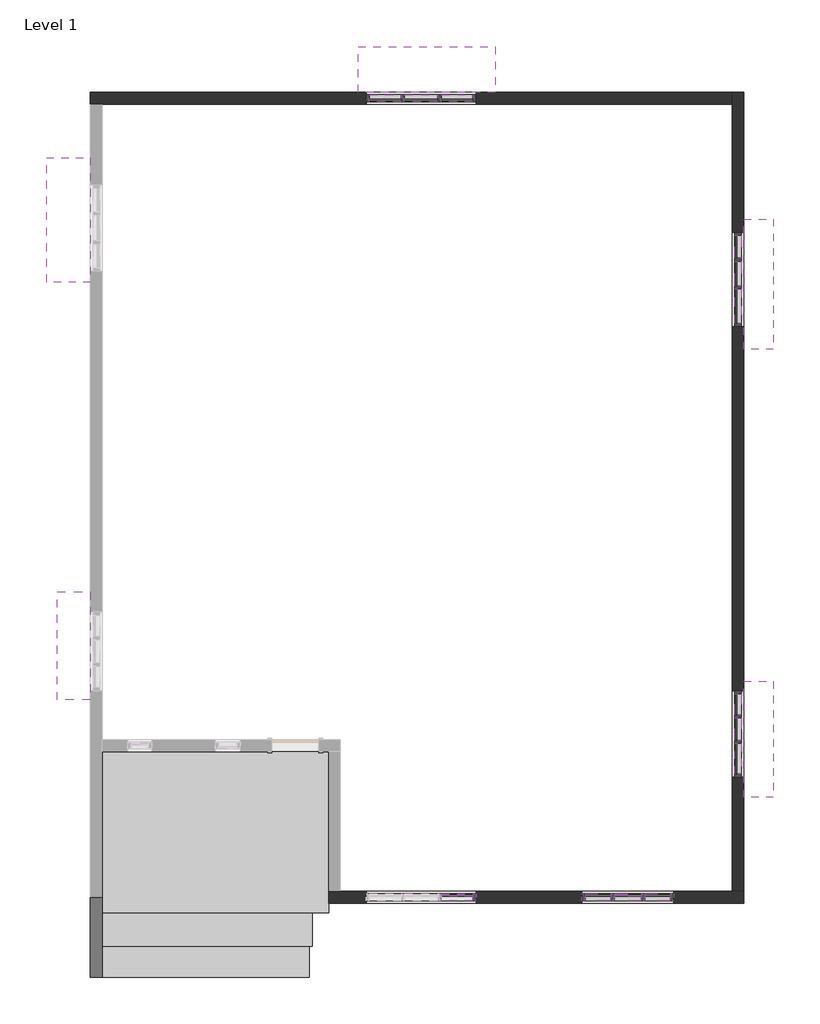
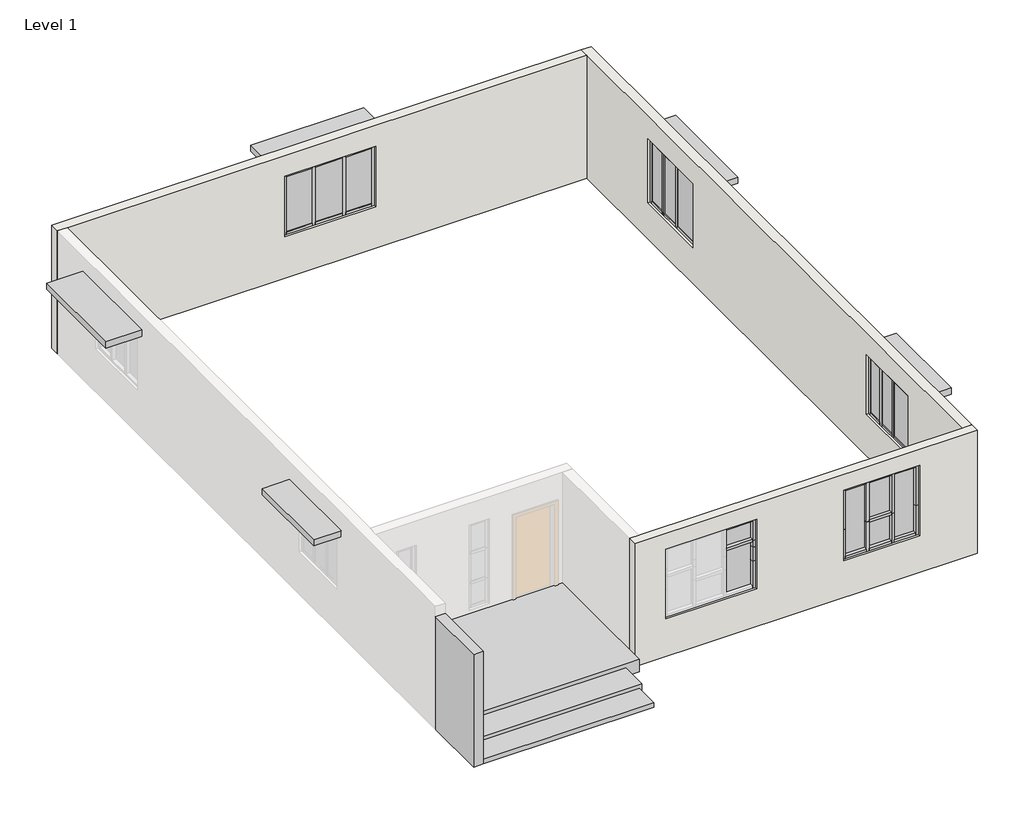
# One storey, part 2 of 2: 51 members, 15 plates, 7 proxies, 3 walls.
"""IFC4 building model written with IfcOpenShell, lengths in millimetres."""

from ifc_helpers import new_model, si_unit, origin, place, context, project, spatial, faceted_brep, transform, mapped, element, save
from components import generic_models_1_generic_models_1_906a804f, generic_models_10_generic_models_10_282af4fe, generic_models_2_generic_models_2_14940448, generic_models_6_generic_models_6_d29c9edd, generic_models_7_generic_models_7_79cca6d0, generic_models_8_generic_models_8_c95dbc8d, generic_models_9_generic_models_9_e403c41d, member_d39130fe, member_be967ef6, member_3f0e0172, member_5215b92c, member_f8dc38bf, member_b3e0441e, member_2caf9219, member_d7af48b5, member_43b2f8c3, member_8ca7f02a, member_b2ed26c7, member_f209f73c, member_fde90c6a, member_7d21ba3d, member_69a911c1, member_1ad5418d, member_e5d39754, member_40abf7f1, member_852981e0, member_2b79973d, member_c33c434a, member_082242e3, member_b4cb8141, member_6fb4a552, member_8bf3bd84, member_143ec642, system_panel_glazed_68735acb, system_panel_glazed_e2a89770, system_panel_glazed_32595814, system_panel_glazed_0cc7d14b, system_panel_glazed_9e372a4a, system_panel_glazed_a8526af5, system_panel_glazed_e1e129e0, system_panel_glazed_32fc5117, system_panel_glazed_c34084c8, system_panel_glazed_d4004c69, system_panel_glazed_e16a1513, system_panel_glazed_7001ef1f, system_panel_glazed_27f6d1d6

model = new_model("IFC4")

# Units and contexts
model_context = context("Model", 3, world=origin())
ifc_project = project(units=[si_unit("LENGTHUNIT", "METRE", prefix="MILLI")], contexts=[model_context])

# Site, building, storey
site = spatial("IfcSite", under=ifc_project)
building = spatial("IfcBuilding", under=site)
storey = spatial("IfcBuildingStorey", under=building, Name="Level 1", Elevation=0.0)

# Proxies
placement = place(None, origin())
generic_models_1_generic_models_1_shape = generic_models_1_generic_models_1_906a804f(model_context)
element("IfcBuildingElementProxy", 1, Name="Generic Models 1 : Generic Models 1", ObjectType="Generic Models 1 : Generic Models 1", at=placement, inside=storey, context=model_context, shape_type="MappedRepresentation", body=[
    mapped(generic_models_1_generic_models_1_shape, transform((0.0, 0.0, 0.0), x_axis=(1.0, 0.0, 0.0), y_axis=(0.0, 1.0, 0.0), z_axis=(0.0, 0.0, 1.0))),
])
generic_models_10_generic_models_10_shape = generic_models_10_generic_models_10_282af4fe(model_context)
element("IfcBuildingElementProxy", 2, Name="Generic Models 10 : Generic Models 10", ObjectType="Generic Models 10 : Generic Models 10", at=placement, inside=storey, context=model_context, shape_type="MappedRepresentation", body=[
    mapped(generic_models_10_generic_models_10_shape, transform((0.0, 0.0, 0.0), x_axis=(1.0, 0.0, 0.0), y_axis=(0.0, 1.0, 0.0), z_axis=(0.0, 0.0, 1.0))),
])
generic_models_2_generic_models_2_shape = generic_models_2_generic_models_2_14940448(model_context)
element("IfcBuildingElementProxy", 3, Name="Generic Models 2 : Generic Models 2", ObjectType="Generic Models 2 : Generic Models 2", at=placement, inside=storey, context=model_context, shape_type="MappedRepresentation", body=[
    mapped(generic_models_2_generic_models_2_shape, transform((0.0, 0.0, 0.0), x_axis=(1.0, 0.0, 0.0), y_axis=(0.0, 1.0, 0.0), z_axis=(0.0, 0.0, 1.0))),
])
generic_models_6_generic_models_6_shape = generic_models_6_generic_models_6_d29c9edd(model_context)
element("IfcBuildingElementProxy", 4, Name="Generic Models 6 : Generic Models 6", ObjectType="Generic Models 6 : Generic Models 6", at=placement, inside=storey, context=model_context, shape_type="MappedRepresentation", body=[
    mapped(generic_models_6_generic_models_6_shape, transform((0.0, 0.0, 0.0), x_axis=(1.0, 0.0, 0.0), y_axis=(0.0, 1.0, 0.0), z_axis=(0.0, 0.0, 1.0))),
])
generic_models_7_generic_models_7_shape = generic_models_7_generic_models_7_79cca6d0(model_context)
element("IfcBuildingElementProxy", 5, Name="Generic Models 7 : Generic Models 7", ObjectType="Generic Models 7 : Generic Models 7", at=placement, inside=storey, context=model_context, shape_type="MappedRepresentation", body=[
    mapped(generic_models_7_generic_models_7_shape, transform((0.0, 0.0, 0.0), x_axis=(1.0, 0.0, 0.0), y_axis=(0.0, 1.0, 0.0), z_axis=(0.0, 0.0, 1.0))),
])
generic_models_8_generic_models_8_shape = generic_models_8_generic_models_8_c95dbc8d(model_context)
element("IfcBuildingElementProxy", 6, Name="Generic Models 8 : Generic Models 8", ObjectType="Generic Models 8 : Generic Models 8", at=placement, inside=storey, context=model_context, shape_type="MappedRepresentation", body=[
    mapped(generic_models_8_generic_models_8_shape, transform((0.0, 0.0, 0.0), x_axis=(1.0, 0.0, 0.0), y_axis=(0.0, 1.0, 0.0), z_axis=(0.0, 0.0, 1.0))),
])
generic_models_9_generic_models_9_shape = generic_models_9_generic_models_9_e403c41d(model_context)
element("IfcBuildingElementProxy", 7, Name="Generic Models 9 : Generic Models 9", ObjectType="Generic Models 9 : Generic Models 9", at=placement, inside=storey, context=model_context, shape_type="MappedRepresentation", body=[
    mapped(generic_models_9_generic_models_9_shape, transform((0.0, 0.0, 0.0), x_axis=(1.0, 0.0, 0.0), y_axis=(0.0, 1.0, 0.0), z_axis=(0.0, 0.0, 1.0))),
])

# Members
member_shape = member_d39130fe(model_context)
element("IfcMember", 8, ObjectType="Rectangular Mullion : 2.5\" x 5\" rectangular", at=placement, inside=storey, context=model_context, shape_type="MappedRepresentation", body=[
    mapped(member_shape, transform((-14378.0161422, -14789.9171312, 1612.541933), x_axis=(1.0, 0.0, 0.0), y_axis=(0.0, -1.0, 0.0), z_axis=(0.0, 0.0, -1.0))),
])
member_2_shape = member_be967ef6(model_context)
element("IfcMember", 9, ObjectType="Rectangular Mullion : 2.5\" x 5\" rectangular", at=placement, inside=storey, context=model_context, shape_type="MappedRepresentation", body=[
    mapped(member_2_shape, transform((-14378.0161422, -14789.9171312, 934.5922675), x_axis=(1.0, 0.0, 0.0), y_axis=(0.0, -1.0, 0.0), z_axis=(0.0, 0.0, -1.0))),
])
member_3_shape = member_3f0e0172(model_context)
element("IfcMember", 10, ObjectType="Rectangular Mullion : 2.5\" x 5\" rectangular", at=placement, inside=storey, context=model_context, shape_type="MappedRepresentation", body=[
    mapped(member_3_shape, transform((-15832.1661422, 678.6828688, 1031.9141224), x_axis=(0.0, 0.0, -1.0), y_axis=(0.0, 1.0, 0.0), z_axis=(1.0, 0.0, 0.0))),
])
element("IfcMember", 11, ObjectType="Rectangular Mullion : 2.5\" x 5\" rectangular", at=placement, inside=storey, context=model_context, shape_type="MappedRepresentation", body=[
    mapped(member_3_shape, transform((-14441.5161422, 678.6828688, 1031.9141224), x_axis=(0.0, 0.0, -1.0), y_axis=(0.0, 1.0, 0.0), z_axis=(1.0, 0.0, 0.0))),
])
element("IfcMember", 12, ObjectType="Rectangular Mullion : 2.5\" x 5\" rectangular", at=placement, inside=storey, context=model_context, shape_type="MappedRepresentation", body=[
    mapped(member_3_shape, transform((-14441.5161422, -14789.9171312, 2663.1790149), x_axis=(0.0, 0.0, 1.0), y_axis=(0.0, -1.0, 0.0), z_axis=(1.0, 0.0, 0.0))),
])
element("IfcMember", 13, ObjectType="Rectangular Mullion : 2.5\" x 5\" rectangular", at=placement, inside=storey, context=model_context, shape_type="MappedRepresentation", body=[
    mapped(member_3_shape, transform((-15057.4661422, 678.6828688, 2530.6098734), x_axis=(0.0, 0.0, 1.0), y_axis=(0.0, 1.0, 0.0), z_axis=(-1.0, 0.0, 0.0))),
])
element("IfcMember", 14, ObjectType="Rectangular Mullion : 2.5\" x 5\" rectangular", at=placement, inside=storey, context=model_context, shape_type="MappedRepresentation", body=[
    mapped(member_3_shape, transform((-16448.1161422, 678.6828688, 2530.6098734), x_axis=(0.0, 0.0, 1.0), y_axis=(0.0, 1.0, 0.0), z_axis=(-1.0, 0.0, 0.0))),
])
member_4_shape = member_5215b92c(model_context)
element("IfcMember", 15, ObjectType="Rectangular Mullion : 2.5\" x 5\" rectangular", at=placement, inside=storey, context=model_context, shape_type="MappedRepresentation", body=[
    mapped(member_4_shape, transform((-15120.9661422, 678.6828688, 1031.9141224), x_axis=(0.0, 0.0, -1.0), y_axis=(0.0, 1.0, 0.0), z_axis=(1.0, 0.0, 0.0))),
])
element("IfcMember", 16, ObjectType="Rectangular Mullion : 2.5\" x 5\" rectangular", at=placement, inside=storey, context=model_context, shape_type="MappedRepresentation", body=[
    mapped(member_4_shape, transform((-15768.6661422, 678.6828688, 2530.6098734), x_axis=(0.0, 0.0, 1.0), y_axis=(0.0, 1.0, 0.0), z_axis=(-1.0, 0.0, 0.0))),
])
member_5_shape = member_f8dc38bf(model_context)
element("IfcMember", 17, ObjectType="Rectangular Mullion : 2.5\" x 5\" rectangular", at=placement, inside=storey, context=model_context, shape_type="MappedRepresentation", body=[
    mapped(member_5_shape, transform((-14441.5161422, -14789.9171312, 2121.0041821), x_axis=(0.0, 0.0, 1.0), y_axis=(0.0, -1.0, 0.0), z_axis=(1.0, 0.0, 0.0))),
])
member_6_shape = member_b3e0441e(model_context)
element("IfcMember", 18, ObjectType="Rectangular Mullion : 2.5\" x 5\" rectangular", at=placement, inside=storey, context=model_context, shape_type="MappedRepresentation", body=[
    mapped(member_6_shape, transform((-14378.0161422, -14789.9171312, 2121.0041821), x_axis=(1.0, 0.0, 0.0), y_axis=(0.0, -1.0, 0.0), z_axis=(0.0, 0.0, -1.0))),
])
member_7_shape = member_2caf9219(model_context)
element("IfcMember", 19, ObjectType="Rectangular Mullion : 2.5\" x 5\" rectangular", at=placement, inside=storey, context=model_context, shape_type="MappedRepresentation", body=[
    mapped(member_7_shape, transform((-14378.0161422, -14789.9171312, 1951.5167658), x_axis=(1.0, 0.0, 0.0), y_axis=(0.0, -1.0, 0.0), z_axis=(0.0, 0.0, -1.0))),
])
member_8_shape = member_d7af48b5(model_context)
element("IfcMember", 20, ObjectType="Rectangular Mullion : 2.5\" x 5\" rectangular", at=placement, inside=storey, context=model_context, shape_type="MappedRepresentation", body=[
    mapped(member_8_shape, transform((-12333.3161422, -14789.9171312, 1648.1799417), x_axis=(-1.0, 0.0, 0.0), y_axis=(0.0, -1.0, 0.0), z_axis=(0.0, 0.0, 1.0))),
])
element("IfcMember", 21, ObjectType="Rectangular Mullion : 2.5\" x 5\" rectangular", at=placement, inside=storey, context=model_context, shape_type="MappedRepresentation", body=[
    mapped(member_8_shape, transform((-10555.3161422, -14789.9171312, 911.5799417), x_axis=(1.0, 0.0, 0.0), y_axis=(0.0, -1.0, 0.0), z_axis=(0.0, 0.0, -1.0))),
])
member_9_shape = member_43b2f8c3(model_context)
element("IfcMember", 22, ObjectType="Rectangular Mullion : 2.5\" x 5\" rectangular", at=placement, inside=storey, context=model_context, shape_type="MappedRepresentation", body=[
    mapped(member_9_shape, transform((-11116.2328089, -14789.9171312, 911.5799417), x_axis=(0.0, 0.0, -1.0), y_axis=(0.0, -1.0, 0.0), z_axis=(-1.0, 0.0, 0.0))),
])
element("IfcMember", 23, ObjectType="Rectangular Mullion : 2.5\" x 5\" rectangular", at=placement, inside=storey, context=model_context, shape_type="MappedRepresentation", body=[
    mapped(member_9_shape, transform((-12269.8161422, -14789.9171312, 911.5799417), x_axis=(0.0, 0.0, -1.0), y_axis=(0.0, -1.0, 0.0), z_axis=(-1.0, 0.0, 0.0))),
])
element("IfcMember", 24, ObjectType="Rectangular Mullion : 2.5\" x 5\" rectangular", at=placement, inside=storey, context=model_context, shape_type="MappedRepresentation", body=[
    mapped(member_9_shape, transform((-11772.3994756, -14789.9171312, 2662.0475339), x_axis=(0.0, 0.0, 1.0), y_axis=(0.0, -1.0, 0.0), z_axis=(1.0, 0.0, 0.0))),
])
element("IfcMember", 25, ObjectType="Rectangular Mullion : 2.5\" x 5\" rectangular", at=placement, inside=storey, context=model_context, shape_type="MappedRepresentation", body=[
    mapped(member_9_shape, transform((-10618.8161422, -14789.9171312, 2662.0475339), x_axis=(0.0, 0.0, 1.0), y_axis=(0.0, -1.0, 0.0), z_axis=(1.0, 0.0, 0.0))),
])
member_10_shape = member_8ca7f02a(model_context)
element("IfcMember", 26, ObjectType="Rectangular Mullion : 2.5\" x 5\" rectangular", at=placement, inside=storey, context=model_context, shape_type="MappedRepresentation", body=[
    mapped(member_10_shape, transform((-11147.9828089, -14789.9171312, 911.5799417), x_axis=(1.0, 0.0, 0.0), y_axis=(0.0, -1.0, 0.0), z_axis=(0.0, 0.0, -1.0))),
])
element("IfcMember", 27, ObjectType="Rectangular Mullion : 2.5\" x 5\" rectangular", at=placement, inside=storey, context=model_context, shape_type="MappedRepresentation", body=[
    mapped(member_10_shape, transform((-11740.6494756, -14789.9171312, 911.5799417), x_axis=(1.0, 0.0, 0.0), y_axis=(0.0, -1.0, 0.0), z_axis=(0.0, 0.0, -1.0))),
])
member_11_shape = member_b2ed26c7(model_context)
element("IfcMember", 28, ObjectType="Rectangular Mullion : 2.5\" x 5\" rectangular", at=placement, inside=storey, context=model_context, shape_type="MappedRepresentation", body=[
    mapped(member_11_shape, transform((-11708.8994756, -14789.9171312, 911.5799417), x_axis=(0.0, 0.0, -1.0), y_axis=(0.0, -1.0, 0.0), z_axis=(-1.0, 0.0, 0.0))),
])
element("IfcMember", 29, ObjectType="Rectangular Mullion : 2.5\" x 5\" rectangular", at=placement, inside=storey, context=model_context, shape_type="MappedRepresentation", body=[
    mapped(member_11_shape, transform((-11179.7328089, -14789.9171312, 2662.0475339), x_axis=(0.0, 0.0, 1.0), y_axis=(0.0, -1.0, 0.0), z_axis=(1.0, 0.0, 0.0))),
])
member_12_shape = member_f209f73c(model_context)
element("IfcMember", 30, ObjectType="Rectangular Mullion : 2.5\" x 5\" rectangular", at=placement, inside=storey, context=model_context, shape_type="MappedRepresentation", body=[
    mapped(member_12_shape, transform((-11179.7328089, -14789.9171312, 1648.1799417), x_axis=(0.0, 0.0, 1.0), y_axis=(0.0, -1.0, 0.0), z_axis=(1.0, 0.0, 0.0))),
])
member_13_shape = member_fde90c6a(model_context)
element("IfcMember", 31, ObjectType="Rectangular Mullion : 2.5\" x 5\" rectangular", at=placement, inside=storey, context=model_context, shape_type="MappedRepresentation", body=[
    mapped(member_13_shape, transform((-11147.9828089, -14789.9171312, 1648.1799417), x_axis=(1.0, 0.0, 0.0), y_axis=(0.0, -1.0, 0.0), z_axis=(0.0, 0.0, -1.0))),
])
element("IfcMember", 32, ObjectType="Rectangular Mullion : 2.5\" x 5\" rectangular", at=placement, inside=storey, context=model_context, shape_type="MappedRepresentation", body=[
    mapped(member_13_shape, transform((-11740.6494756, -14789.9171312, 1648.1799417), x_axis=(1.0, 0.0, 0.0), y_axis=(0.0, -1.0, 0.0), z_axis=(0.0, 0.0, -1.0))),
])
member_14_shape = member_7d21ba3d(model_context)
element("IfcMember", 33, ObjectType="Rectangular Mullion : 2.5\" x 5\" rectangular", at=placement, inside=storey, context=model_context, shape_type="MappedRepresentation", body=[
    mapped(member_14_shape, transform((-12333.3161422, -14789.9171312, 2662.0475339), x_axis=(-1.0, 0.0, 0.0), y_axis=(0.0, -1.0, 0.0), z_axis=(0.0, 0.0, 1.0))),
])
element("IfcMember", 34, ObjectType="Rectangular Mullion : 2.5\" x 5\" rectangular", at=placement, inside=storey, context=model_context, shape_type="MappedRepresentation", body=[
    mapped(member_14_shape, transform((-10555.3161422, -14789.9171312, 1648.1799417), x_axis=(1.0, 0.0, 0.0), y_axis=(0.0, -1.0, 0.0), z_axis=(0.0, 0.0, -1.0))),
])
member_15_shape = member_69a911c1(model_context)
element("IfcMember", 35, ObjectType="Rectangular Mullion : 2.5\" x 5\" rectangular", at=placement, inside=storey, context=model_context, shape_type="MappedRepresentation", body=[
    mapped(member_15_shape, transform((-9310.7161422, -11316.4671312, 2505.560435), x_axis=(0.0, 0.0, 1.0), y_axis=(1.0, 0.0, 0.0), z_axis=(0.0, 1.0, 0.0))),
])
member_16_shape = member_1ad5418d(model_context)
element("IfcMember", 36, ObjectType="Rectangular Mullion : 2.5\" x 5\" rectangular", at=placement, inside=storey, context=model_context, shape_type="MappedRepresentation", body=[
    mapped(member_16_shape, transform((-9310.7161422, -10852.9171312, 2505.560435), x_axis=(0.0, 0.0, 1.0), y_axis=(1.0, 0.0, 0.0), z_axis=(0.0, 1.0, 0.0))),
])
member_17_shape = member_e5d39754(model_context)
element("IfcMember", 37, ObjectType="Rectangular Mullion : 2.5\" x 5\" rectangular", at=placement, inside=storey, context=model_context, shape_type="MappedRepresentation", body=[
    mapped(member_17_shape, transform((-9310.7161422, -11811.7671312, 2505.560435), x_axis=(0.0, 0.0, 1.0), y_axis=(1.0, 0.0, 0.0), z_axis=(0.0, 1.0, 0.0))),
])
member_18_shape = member_40abf7f1(model_context)
element("IfcMember", 38, ObjectType="Rectangular Mullion : 2.5\" x 5\" rectangular", at=placement, inside=storey, context=model_context, shape_type="MappedRepresentation", body=[
    mapped(member_18_shape, transform((-9310.7161422, -11780.0171312, 1029.7783149), x_axis=(0.0, 1.0, 0.0), y_axis=(1.0, 0.0, 0.0), z_axis=(0.0, 0.0, -1.0))),
])
element("IfcMember", 39, ObjectType="Rectangular Mullion : 2.5\" x 5\" rectangular", at=placement, inside=storey, context=model_context, shape_type="MappedRepresentation", body=[
    mapped(member_18_shape, transform((-9310.7161422, -11284.7171312, 1029.7783149), x_axis=(0.0, 1.0, 0.0), y_axis=(1.0, 0.0, 0.0), z_axis=(0.0, 0.0, -1.0))),
])
element("IfcMember", 40, ObjectType="Rectangular Mullion : 2.5\" x 5\" rectangular", at=placement, inside=storey, context=model_context, shape_type="MappedRepresentation", body=[
    mapped(member_16_shape, transform((-9310.7161422, -11252.9671312, 1029.7783149), x_axis=(0.0, 0.0, -1.0), y_axis=(1.0, 0.0, 0.0), z_axis=(0.0, -1.0, 0.0))),
])
element("IfcMember", 41, ObjectType="Rectangular Mullion : 2.5\" x 5\" rectangular", at=placement, inside=storey, context=model_context, shape_type="MappedRepresentation", body=[
    mapped(member_15_shape, transform((-9310.7161422, -11748.2671312, 1029.7783149), x_axis=(0.0, 0.0, -1.0), y_axis=(1.0, 0.0, 0.0), z_axis=(0.0, -1.0, 0.0))),
])
element("IfcMember", 42, ObjectType="Rectangular Mullion : 2.5\" x 5\" rectangular", at=placement, inside=storey, context=model_context, shape_type="MappedRepresentation", body=[
    mapped(member_17_shape, transform((-9310.7161422, -12402.3171312, 1029.7783149), x_axis=(0.0, 0.0, -1.0), y_axis=(1.0, 0.0, 0.0), z_axis=(0.0, -1.0, 0.0))),
])
member_19_shape = member_852981e0(model_context)
element("IfcMember", 43, ObjectType="Rectangular Mullion : 2.5\" x 5\" rectangular", at=placement, inside=storey, context=model_context, shape_type="MappedRepresentation", body=[
    mapped(member_19_shape, transform((-9310.7161422, -10789.4171312, 1029.7783149), x_axis=(0.0, 1.0, 0.0), y_axis=(1.0, 0.0, 0.0), z_axis=(0.0, 0.0, -1.0))),
])
element("IfcMember", 44, ObjectType="Rectangular Mullion : 2.5\" x 5\" rectangular", at=placement, inside=storey, context=model_context, shape_type="MappedRepresentation", body=[
    mapped(member_19_shape, transform((-9310.7161422, -12465.8171312, 2505.560435), x_axis=(0.0, -1.0, 0.0), y_axis=(1.0, 0.0, 0.0), z_axis=(0.0, 0.0, 1.0))),
])
member_20_shape = member_2b79973d(model_context)
element("IfcMember", 45, ObjectType="Rectangular Mullion : 2.5\" x 5\" rectangular", at=placement, inside=storey, context=model_context, shape_type="MappedRepresentation", body=[
    mapped(member_20_shape, transform((-9310.7161422, -2477.2671312, 2477.8166854), x_axis=(0.0, 0.0, 1.0), y_axis=(1.0, 0.0, 0.0), z_axis=(0.0, 1.0, 0.0))),
])
member_21_shape = member_c33c434a(model_context)
element("IfcMember", 46, ObjectType="Rectangular Mullion : 2.5\" x 5\" rectangular", at=placement, inside=storey, context=model_context, shape_type="MappedRepresentation", body=[
    mapped(member_21_shape, transform((-9310.7161422, -3010.6671312, 2477.8166854), x_axis=(0.0, 0.0, 1.0), y_axis=(1.0, 0.0, 0.0), z_axis=(0.0, 1.0, 0.0))),
])
member_22_shape = member_082242e3(model_context)
element("IfcMember", 47, ObjectType="Rectangular Mullion : 2.5\" x 5\" rectangular", at=placement, inside=storey, context=model_context, shape_type="MappedRepresentation", body=[
    mapped(member_22_shape, transform((-9310.7161422, -2445.5171312, 891.689976), x_axis=(0.0, 1.0, 0.0), y_axis=(1.0, 0.0, 0.0), z_axis=(0.0, 0.0, -1.0))),
])
element("IfcMember", 48, ObjectType="Rectangular Mullion : 2.5\" x 5\" rectangular", at=placement, inside=storey, context=model_context, shape_type="MappedRepresentation", body=[
    mapped(member_22_shape, transform((-9310.7161422, -2978.9171312, 891.689976), x_axis=(0.0, 1.0, 0.0), y_axis=(1.0, 0.0, 0.0), z_axis=(0.0, 0.0, -1.0))),
])
element("IfcMember", 49, ObjectType="Rectangular Mullion : 2.5\" x 5\" rectangular", at=placement, inside=storey, context=model_context, shape_type="MappedRepresentation", body=[
    mapped(member_20_shape, transform((-9310.7161422, -2947.1671312, 891.689976), x_axis=(0.0, 0.0, -1.0), y_axis=(1.0, 0.0, 0.0), z_axis=(0.0, -1.0, 0.0))),
])
element("IfcMember", 50, ObjectType="Rectangular Mullion : 2.5\" x 5\" rectangular", at=placement, inside=storey, context=model_context, shape_type="MappedRepresentation", body=[
    mapped(member_21_shape, transform((-9310.7161422, -3677.4171312, 891.689976), x_axis=(0.0, 0.0, -1.0), y_axis=(1.0, 0.0, 0.0), z_axis=(0.0, -1.0, 0.0))),
])
member_23_shape = member_b4cb8141(model_context)
element("IfcMember", 51, ObjectType="Rectangular Mullion : 2.5\" x 5\" rectangular", at=placement, inside=storey, context=model_context, shape_type="MappedRepresentation", body=[
    mapped(member_23_shape, transform((-9310.7161422, -3740.9171312, 2477.8166854), x_axis=(0.0, -1.0, 0.0), y_axis=(1.0, 0.0, 0.0), z_axis=(0.0, 0.0, 1.0))),
])
member_24_shape = member_6fb4a552(model_context)
element("IfcMember", 52, ObjectType="Rectangular Mullion : 2.5\" x 5\" rectangular", at=placement, inside=storey, context=model_context, shape_type="MappedRepresentation", body=[
    mapped(member_24_shape, transform((-9310.7161422, -1975.6171312, 2477.8166854), x_axis=(0.0, 0.0, 1.0), y_axis=(1.0, 0.0, 0.0), z_axis=(0.0, 1.0, 0.0))),
])
element("IfcMember", 53, ObjectType="Rectangular Mullion : 2.5\" x 5\" rectangular", at=placement, inside=storey, context=model_context, shape_type="MappedRepresentation", body=[
    mapped(member_24_shape, transform((-9310.7161422, -2413.7671312, 891.689976), x_axis=(0.0, 0.0, -1.0), y_axis=(1.0, 0.0, 0.0), z_axis=(0.0, -1.0, 0.0))),
])
element("IfcMember", 54, ObjectType="Rectangular Mullion : 2.5\" x 5\" rectangular", at=placement, inside=storey, context=model_context, shape_type="MappedRepresentation", body=[
    mapped(member_23_shape, transform((-9310.7161422, -1912.1171312, 891.689976), x_axis=(0.0, 1.0, 0.0), y_axis=(1.0, 0.0, 0.0), z_axis=(0.0, 0.0, -1.0))),
])
member_25_shape = member_8bf3bd84(model_context)
element("IfcMember", 55, ObjectType="Rectangular Mullion : 2.5\" x 5\" rectangular", at=placement, inside=storey, context=model_context, shape_type="MappedRepresentation", body=[
    mapped(member_25_shape, transform((-15089.2161422, 678.6828688, 1031.9141224), x_axis=(-1.0, 0.0, 0.0), y_axis=(0.0, 1.0, 0.0), z_axis=(0.0, 0.0, -1.0))),
])
element("IfcMember", 56, ObjectType="Rectangular Mullion : 2.5\" x 5\" rectangular", at=placement, inside=storey, context=model_context, shape_type="MappedRepresentation", body=[
    mapped(member_25_shape, transform((-15800.4161422, 678.6828688, 1031.9141224), x_axis=(-1.0, 0.0, 0.0), y_axis=(0.0, 1.0, 0.0), z_axis=(0.0, 0.0, -1.0))),
])
member_26_shape = member_143ec642(model_context)
element("IfcMember", 57, ObjectType="Rectangular Mullion : 2.5\" x 5\" rectangular", at=placement, inside=storey, context=model_context, shape_type="MappedRepresentation", body=[
    mapped(member_26_shape, transform((-14378.0161422, 678.6828688, 2530.6098734), x_axis=(1.0, 0.0, 0.0), y_axis=(0.0, 1.0, 0.0), z_axis=(0.0, 0.0, 1.0))),
])
element("IfcMember", 58, ObjectType="Rectangular Mullion : 2.5\" x 5\" rectangular", at=placement, inside=storey, context=model_context, shape_type="MappedRepresentation", body=[
    mapped(member_26_shape, transform((-16511.6161422, 678.6828688, 1031.9141224), x_axis=(-1.0, 0.0, 0.0), y_axis=(0.0, 1.0, 0.0), z_axis=(0.0, 0.0, -1.0))),
])

# Plates
system_panel_glazed_shape = system_panel_glazed_68735acb(model_context)
element("IfcPlate", 59, ObjectType="System Panel : Glazed", at=placement, inside=storey, context=model_context, shape_type="MappedRepresentation", body=[
    mapped(system_panel_glazed_shape, transform((-14749.4911422, -14789.9171312, 998.0922675), x_axis=(1.0, 0.0, 0.0), y_axis=(0.0, 1.0, 0.0), z_axis=(0.0, 0.0, 1.0))),
])
system_panel_glazed_2_shape = system_panel_glazed_e2a89770(model_context)
element("IfcPlate", 60, ObjectType="System Panel : Glazed", at=placement, inside=storey, context=model_context, shape_type="MappedRepresentation", body=[
    mapped(system_panel_glazed_2_shape, transform((-14749.4911422, -14789.9171312, 2152.7541821), x_axis=(1.0, 0.0, 0.0), y_axis=(0.0, 1.0, 0.0), z_axis=(0.0, 0.0, 1.0))),
])
system_panel_glazed_3_shape = system_panel_glazed_32595814(model_context)
element("IfcPlate", 61, ObjectType="System Panel : Glazed", at=placement, inside=storey, context=model_context, shape_type="MappedRepresentation", body=[
    mapped(system_panel_glazed_3_shape, transform((-11444.3161422, -14789.9171312, 975.0799417), x_axis=(1.0, 0.0, 0.0), y_axis=(0.0, 1.0, 0.0), z_axis=(0.0, 0.0, 1.0))),
])
system_panel_glazed_4_shape = system_panel_glazed_0cc7d14b(model_context)
element("IfcPlate", 62, ObjectType="System Panel : Glazed", at=placement, inside=storey, context=model_context, shape_type="MappedRepresentation", body=[
    mapped(system_panel_glazed_4_shape, transform((-12021.1078089, -14789.9171312, 975.0799417), x_axis=(1.0, 0.0, 0.0), y_axis=(0.0, 1.0, 0.0), z_axis=(0.0, 0.0, 1.0))),
])
element("IfcPlate", 63, ObjectType="System Panel : Glazed", at=placement, inside=storey, context=model_context, shape_type="MappedRepresentation", body=[
    mapped(system_panel_glazed_4_shape, transform((-10867.5244756, -14789.9171312, 975.0799417), x_axis=(1.0, 0.0, 0.0), y_axis=(0.0, 1.0, 0.0), z_axis=(0.0, 0.0, 1.0))),
])
system_panel_glazed_5_shape = system_panel_glazed_9e372a4a(model_context)
element("IfcPlate", 64, ObjectType="System Panel : Glazed", at=placement, inside=storey, context=model_context, shape_type="MappedRepresentation", body=[
    mapped(system_panel_glazed_5_shape, transform((-11444.3161422, -14789.9171312, 1679.9299417), x_axis=(1.0, 0.0, 0.0), y_axis=(0.0, 1.0, 0.0), z_axis=(0.0, 0.0, 1.0))),
])
system_panel_glazed_6_shape = system_panel_glazed_a8526af5(model_context)
element("IfcPlate", 65, ObjectType="System Panel : Glazed", at=placement, inside=storey, context=model_context, shape_type="MappedRepresentation", body=[
    mapped(system_panel_glazed_6_shape, transform((-9310.7161422, -12107.0421312, 1093.2783149), x_axis=(0.0, 1.0, 0.0), y_axis=(-1.0, 0.0, 0.0), z_axis=(0.0, 0.0, 1.0))),
])
system_panel_glazed_7_shape = system_panel_glazed_e1e129e0(model_context)
element("IfcPlate", 66, ObjectType="System Panel : Glazed", at=placement, inside=storey, context=model_context, shape_type="MappedRepresentation", body=[
    mapped(system_panel_glazed_7_shape, transform((-9310.7161422, -11532.3671312, 1093.2783149), x_axis=(0.0, 1.0, 0.0), y_axis=(-1.0, 0.0, 0.0), z_axis=(0.0, 0.0, 1.0))),
])
system_panel_glazed_8_shape = system_panel_glazed_32fc5117(model_context)
element("IfcPlate", 67, ObjectType="System Panel : Glazed", at=placement, inside=storey, context=model_context, shape_type="MappedRepresentation", body=[
    mapped(system_panel_glazed_8_shape, transform((-9310.7161422, -11052.9421312, 1093.2783149), x_axis=(0.0, 1.0, 0.0), y_axis=(-1.0, 0.0, 0.0), z_axis=(0.0, 0.0, 1.0))),
])
system_panel_glazed_9_shape = system_panel_glazed_c34084c8(model_context)
element("IfcPlate", 68, ObjectType="System Panel : Glazed", at=placement, inside=storey, context=model_context, shape_type="MappedRepresentation", body=[
    mapped(system_panel_glazed_9_shape, transform((-9310.7161422, -3344.0421312, 955.189976), x_axis=(0.0, 1.0, 0.0), y_axis=(-1.0, 0.0, 0.0), z_axis=(0.0, 0.0, 1.0))),
])
system_panel_glazed_10_shape = system_panel_glazed_d4004c69(model_context)
element("IfcPlate", 69, ObjectType="System Panel : Glazed", at=placement, inside=storey, context=model_context, shape_type="MappedRepresentation", body=[
    mapped(system_panel_glazed_10_shape, transform((-9310.7161422, -2712.2171312, 955.189976), x_axis=(0.0, 1.0, 0.0), y_axis=(-1.0, 0.0, 0.0), z_axis=(0.0, 0.0, 1.0))),
])
system_panel_glazed_11_shape = system_panel_glazed_e16a1513(model_context)
element("IfcPlate", 70, ObjectType="System Panel : Glazed", at=placement, inside=storey, context=model_context, shape_type="MappedRepresentation", body=[
    mapped(system_panel_glazed_11_shape, transform((-9310.7161422, -2194.6921312, 955.189976), x_axis=(0.0, 1.0, 0.0), y_axis=(-1.0, 0.0, 0.0), z_axis=(0.0, 0.0, 1.0))),
])
system_panel_glazed_12_shape = system_panel_glazed_7001ef1f(model_context)
element("IfcPlate", 71, ObjectType="System Panel : Glazed", at=placement, inside=storey, context=model_context, shape_type="MappedRepresentation", body=[
    mapped(system_panel_glazed_12_shape, transform((-14749.4911422, 678.6828688, 1095.4141224), x_axis=(-1.0, 0.0, 0.0), y_axis=(0.0, -1.0, 0.0), z_axis=(0.0, 0.0, 1.0))),
])
element("IfcPlate", 72, ObjectType="System Panel : Glazed", at=placement, inside=storey, context=model_context, shape_type="MappedRepresentation", body=[
    mapped(system_panel_glazed_12_shape, transform((-16140.1411422, 678.6828688, 1095.4141224), x_axis=(-1.0, 0.0, 0.0), y_axis=(0.0, -1.0, 0.0), z_axis=(0.0, 0.0, 1.0))),
])
system_panel_glazed_13_shape = system_panel_glazed_27f6d1d6(model_context)
element("IfcPlate", 73, ObjectType="System Panel : Glazed", at=placement, inside=storey, context=model_context, shape_type="MappedRepresentation", body=[
    mapped(system_panel_glazed_13_shape, transform((-15444.8161422, 678.6828688, 1095.4141224), x_axis=(-1.0, 0.0, 0.0), y_axis=(0.0, -1.0, 0.0), z_axis=(0.0, 0.0, 1.0))),
])

# Walls
element("IfcWall", 74, ObjectType="9\"", at=placement, inside=storey, context=model_context, shape_type="Brep", body=[
    faceted_brep([(-9196.4161422, -14675.6171312, 0.0), (-9196.4161422, 792.9828688, 0.0), (-9196.4161422, 792.9828688, 3048.0), (-9196.4161422, -14675.6171312, 3048.0), (-9196.4161422, -12465.8171312, 1029.7783149), (-9196.4161422, -12465.8171312, 2505.560435), (-9196.4161422, -10789.4171312, 2505.560435), (-9196.4161422, -10789.4171312, 1029.7783149), (-9196.4161422, -3740.9171312, 891.689976), (-9196.4161422, -3740.9171312, 2477.8166854), (-9196.4161422, -1912.1171312, 2477.8166854), (-9196.4161422, -1912.1171312, 891.689976), (-9425.0161422, 792.9828688, 0.0), (-9425.0161422, 564.3828688, 0.0), (-9425.0161422, -14675.6171312, 0.0), (-9425.0161422, -14675.6171312, 3048.0), (-9425.0161422, 564.3828688, 3048.0), (-9425.0161422, 792.9828688, 3048.0), (-9425.0161422, -12465.8171312, 2505.560435), (-9425.0161422, -12465.8171312, 1029.7783149), (-9425.0161422, -10789.4171312, 1029.7783149), (-9425.0161422, -10789.4171312, 2505.560435), (-9425.0161422, -3740.9171312, 2477.8166854), (-9425.0161422, -3740.9171312, 891.689976), (-9425.0161422, -1912.1171312, 891.689976), (-9425.0161422, -1912.1171312, 2477.8166854)], [[[0, 1, 2, 3], [4, 5, 6, 7], [8, 9, 10, 11]], [[12, 13, 14, 15, 16, 17], [18, 19, 20, 21], [22, 23, 24, 25]], [[1, 0, 14, 13, 12]], [[3, 2, 17, 16, 15]], [[0, 3, 15, 14]], [[2, 1, 12, 17]], [[18, 5, 4, 19]], [[5, 18, 21, 6]], [[6, 21, 20, 7]], [[19, 4, 7, 20]], [[8, 23, 22, 9]], [[9, 22, 25, 10]], [[10, 25, 24, 11]], [[23, 8, 11, 24]]]),
])
element("IfcWall", 75, ObjectType="9\"", at=placement, inside=storey, context=model_context, shape_type="Brep", body=[
    faceted_brep([(-9425.0161422, 792.9828688, 0.0), (-21845.6161422, 792.9828688, 0.0), (-21845.6161422, 792.9828688, 3048.0), (-9425.0161422, 792.9828688, 3048.0), (-14378.0161422, 792.9828688, 1031.9141224), (-14378.0161422, 792.9828688, 2530.6098734), (-16511.6161422, 792.9828688, 2530.6098734), (-16511.6161422, 792.9828688, 1031.9141224), (-21845.6161422, 564.3828688, 0.0), (-21617.0161422, 564.3828688, 0.0), (-9425.0161422, 564.3828688, 0.0), (-9425.0161422, 564.3828688, 3048.0), (-21617.0161422, 564.3828688, 3048.0), (-21845.6161422, 564.3828688, 3048.0), (-14378.0161422, 564.3828688, 2530.6098734), (-14378.0161422, 564.3828688, 1031.9141224), (-16511.6161422, 564.3828688, 1031.9141224), (-16511.6161422, 564.3828688, 2530.6098734)], [[[0, 1, 2, 3], [4, 5, 6, 7]], [[8, 9, 10, 11, 12, 13], [14, 15, 16, 17]], [[1, 0, 10, 9, 8]], [[3, 2, 13, 12, 11]], [[0, 3, 11, 10]], [[2, 1, 8, 13]], [[4, 15, 14, 5]], [[5, 14, 17, 6]], [[6, 17, 16, 7]], [[15, 4, 7, 16]]]),
])
element("IfcWall", 76, ObjectType="9\"", at=placement, inside=storey, context=model_context, shape_type="Brep", body=[
    faceted_brep([(-17235.5161422, -14904.2171312, 0.0), (-9196.4161422, -14904.2171312, 0.0), (-9196.4161422, -14904.2171312, 3048.0), (-17235.5161422, -14904.2171312, 3048.0), (-16511.6161422, -14904.2171312, 934.5922675), (-16511.6161422, -14904.2171312, 2663.1790149), (-14378.0161422, -14904.2171312, 2663.1790149), (-14378.0161422, -14904.2171312, 934.5922675), (-12333.3161422, -14904.2171312, 911.5799417), (-12333.3161422, -14904.2171312, 2662.0475339), (-10555.3161422, -14904.2171312, 2662.0475339), (-10555.3161422, -14904.2171312, 911.5799417), (-9196.4161422, -14675.6171312, 0.0), (-9425.0161422, -14675.6171312, 0.0), (-17006.9161422, -14675.6171312, 0.0), (-17235.5161422, -14675.6171312, 0.0), (-17235.5161422, -14675.6171312, 3048.0), (-17006.9161422, -14675.6171312, 3048.0), (-9425.0161422, -14675.6171312, 3048.0), (-9196.4161422, -14675.6171312, 3048.0), (-16511.6161422, -14675.6171312, 2663.1790149), (-16511.6161422, -14675.6171312, 934.5922675), (-14378.0161422, -14675.6171312, 934.5922675), (-14378.0161422, -14675.6171312, 2663.1790149), (-12333.3161422, -14675.6171312, 2662.0475339), (-12333.3161422, -14675.6171312, 911.5799417), (-10555.3161422, -14675.6171312, 911.5799417), (-10555.3161422, -14675.6171312, 2662.0475339)], [[[0, 1, 2, 3], [4, 5, 6, 7], [8, 9, 10, 11]], [[12, 13, 14, 15, 16, 17, 18, 19], [20, 21, 22, 23], [24, 25, 26, 27]], [[2, 1, 12, 19]], [[20, 5, 4, 21]], [[5, 20, 23, 6]], [[6, 23, 22, 7]], [[21, 4, 7, 22]], [[8, 25, 24, 9]], [[9, 24, 27, 10]], [[10, 27, 26, 11]], [[25, 8, 11, 26]], [[1, 0, 15, 14, 13, 12]], [[3, 2, 19, 18, 17, 16]], [[0, 3, 16, 15]]]),
])

save(model, "model.ifc")

# Revit data of these elements
# Type "Rectangular Mullion : 2.5\" x 5\" rectangular"
#   built-in parameter 1007304 = 0.416667 (stored number, unit not read)
#   built-in parameter 1007301 = 0.104167 (stored number, unit not read)
#   built-in parameter 1007300 = 0.104167 (stored number, unit not read)
# Type "System Panel : Glazed"
#   Construction Type Id = "GSP4R"
#   Analytic Construction = "1/8 in Pilkington single glazing"
#   Visual Light Transmittance = 0.9
#   Solar Heat Gain Coefficient = 0.86
#   Heat Transfer Coefficient (U) = 1.18115 BTU/(h·ft²·°F)
#   Define Thermal Properties by = 1
# Type "9\""
#   Assembly Code = "B2010"
#   Layers, outside or top first: 0' - 9" no material (function 1)
# Element 1 (IfcBuildingElementProxy, "Generic Models 1 : Generic Models 1")
#   Phase Created = New Construction
# Element 2 (IfcBuildingElementProxy, "Generic Models 10 : Generic Models 10")
#   Phase Created = New Construction
# Element 3 (IfcBuildingElementProxy, "Generic Models 2 : Generic Models 2")
#   Phase Created = New Construction
# Element 4 (IfcBuildingElementProxy, "Generic Models 6 : Generic Models 6")
#   Phase Created = New Construction
# Element 5 (IfcBuildingElementProxy, "Generic Models 7 : Generic Models 7")
#   Phase Created = New Construction
# Element 6 (IfcBuildingElementProxy, "Generic Models 8 : Generic Models 8")
#   Phase Created = New Construction
# Element 7 (IfcBuildingElementProxy, "Generic Models 9 : Generic Models 9")
#   Phase Created = New Construction
# Elements 8, 9, 10, 11, 12, 13, 14, 15, 16, 17, 18, 19, 20, 21, 22, 23, 24, 25, 26, 27, 28, 29, 30, 31, 32, 33, 34, 35, 36, 37, 38, 39, 40, 41, 42, 43, 44, 45, 46, 47, 48, 49, 50, 51, 52, 53, 54, 55, 56, 57, 58 (IfcMember, "Rectangular Mullion : 2.5\" x 5\" rectangular")
#   Phase Created = New Construction
#   Materials on its faces: "Aluminum"
# Elements 59, 60, 61, 62, 63, 64, 65, 66, 67, 68, 69, 70, 71, 72, 73 (IfcPlate, "System Panel : Glazed")
#   Phase Created = New Construction
#   Materials on its faces: "Glass"
# Elements 74, 75, 76 (IfcWall, "9\"")
#   Top Offset = 0' - 0"
#   Base Offset = 0' - 0"
#   Unconnected Height = 10' - 0"
#   wall height = 10' - 0"
#   Phase Created = New Construction
#   Base Constraint = Level 1
#   Materials on its faces: "Default Wall"
# Materials
#   "Aluminum": class "Metal", colour RGB 247 247 247, transparency 0, Description = "Aluminum 6061", Cost = 0
#   "Glass": class "Glass", colour RGB 0 128 192, transparency 0.75, Description = "Soda Lime Glass", Cost = 0
#   "Default Wall": colour RGB 128 128 128, transparency 0, Cost = 0
